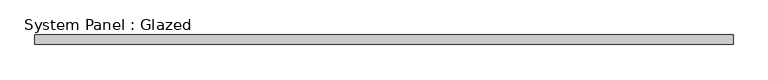
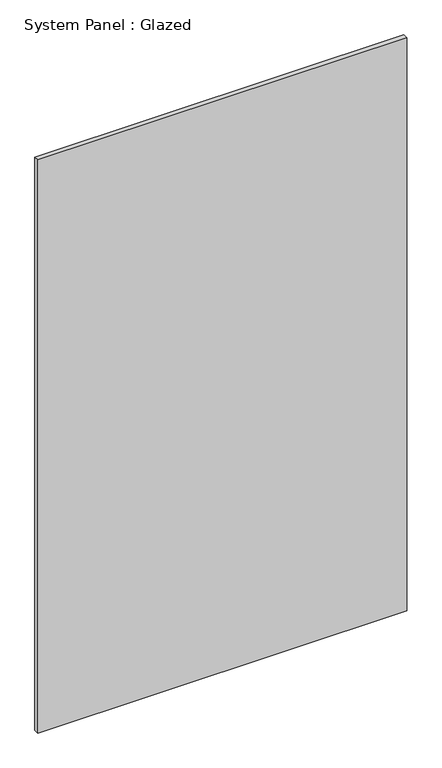
"""IFC4 building model written with IfcOpenShell, lengths in millimetres: plate geometry, System Panel : Glazed."""

from ifc_helpers import new_model, si_unit, origin, origin_with_axes, place, context, project, spatial, polyline, outline, extrude, source, transform, mapped, element, save


def system_panel_glazed_6ac8334b(model_context):
    return source(origin(), model_context, "Body", "SweptSolid", [
        extrude(outline(polyline([(913.2037359, 24.5), (-913.2037359, 24.5), (-913.2037359, 49.5), (913.2037359, 49.5), (913.2037359, 24.5)])), origin_with_axes(), (0.0, 0.0, 1.0), 3000.0),
    ])


if __name__ == "__main__":
    model = new_model("IFC4")
    model_context = context("Model", 3, world=origin())
    ifc_project = project(units=[si_unit("LENGTHUNIT", "METRE", prefix="MILLI")], contexts=[model_context])
    site = spatial("IfcSite", under=ifc_project)
    building = spatial("IfcBuilding", under=site)
    placement = place(None, origin())
    system_panel_glazed_shape = system_panel_glazed_6ac8334b(model_context)
    element("IfcPlate", 1, ObjectType="System Panel : Glazed", at=placement, inside=building, context=model_context, shape_type="MappedRepresentation", body=[
        mapped(system_panel_glazed_shape, transform((0.0, 0.0, 0.0), x_axis=(1.0, 0.0, 0.0), y_axis=(0.0, 1.0, 0.0), z_axis=(0.0, 0.0, 1.0))),
    ])
    save(model, "model.ifc")

# Revit data of these elements
# Type "System Panel : Glazed"
#   Keynote = "H11"
#   Construction Type Id = "GSP4R"
#   Analytic Construction = "1/8 in Pilkington single glazing"
#   Visual Light Transmittance = 0.9
#   Solar Heat Gain Coefficient = 0.86
#   Heat Transfer Coefficient (U) = 6.7069 W/(m²·K)
#   Define Thermal Properties by = 1
# Element 1 (IfcPlate, "System Panel : Glazed")
#   Materials on its faces: "Glass"
# Materials
#   "Glass": class "Glass", colour RGB 0 128 192, transparency 0.9, Description = "Soda Lime Glass", Cost = 0
